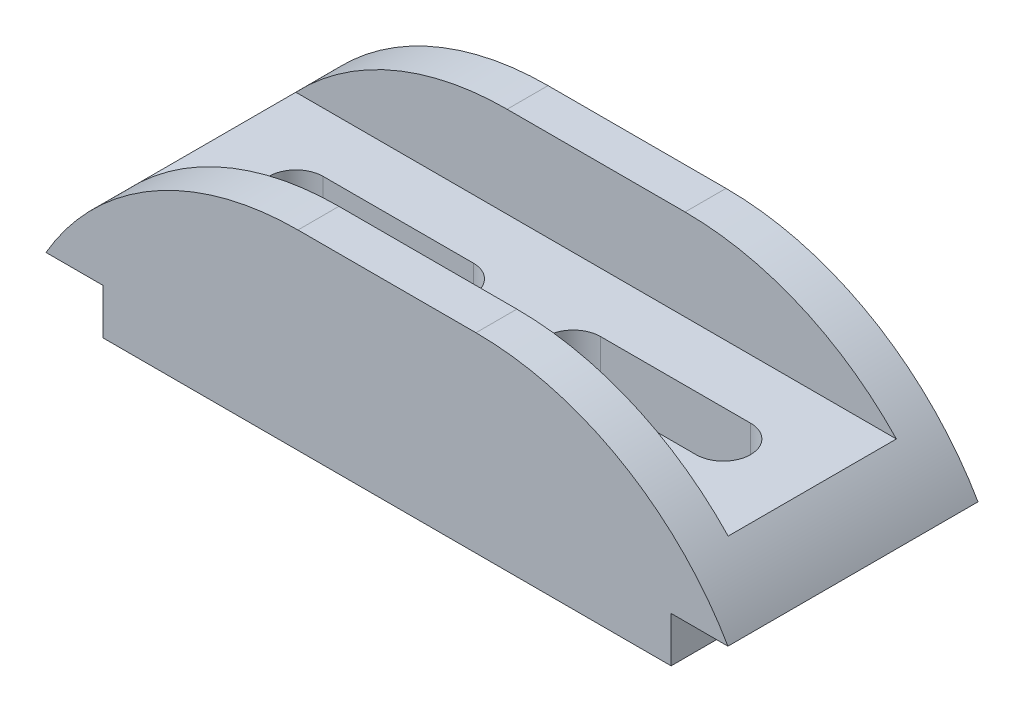
ISO-10303-21;
HEADER;
FILE_DESCRIPTION(('STEP AP214'),'2;1');
FILE_NAME('part.step','',(''),(''),'','','');
FILE_SCHEMA(('AUTOMOTIVE_DESIGN { 1 0 10303 214 1 1 1 1 }'));
ENDSEC;
DATA;
#1=APPLICATION_CONTEXT('core data for automotive mechanical design processes');
#2=APPLICATION_PROTOCOL_DEFINITION('international standard','automotive_design',2000,#1);
#3=PRODUCT_CONTEXT('',#1,'mechanical');
#4=PRODUCT('Part','Part','',(#3));
#5=PRODUCT_RELATED_PRODUCT_CATEGORY('part','',(#4));
#6=PRODUCT_DEFINITION_FORMATION('','',#4);
#7=PRODUCT_DEFINITION_CONTEXT('part definition',#1,'design');
#8=PRODUCT_DEFINITION('design','',#6,#7);
#9=PRODUCT_DEFINITION_SHAPE('','',#8);
#10=(LENGTH_UNIT() NAMED_UNIT(*) SI_UNIT(.MILLI.,.METRE.));
#11=(NAMED_UNIT(*) PLANE_ANGLE_UNIT() SI_UNIT($,.RADIAN.));
#12=(NAMED_UNIT(*) SI_UNIT($,.STERADIAN.) SOLID_ANGLE_UNIT());
#13=UNCERTAINTY_MEASURE_WITH_UNIT(LENGTH_MEASURE(1.E-05),#10,'distance_accuracy_value','');
#14=(GEOMETRIC_REPRESENTATION_CONTEXT(3) GLOBAL_UNCERTAINTY_ASSIGNED_CONTEXT((#13)) GLOBAL_UNIT_ASSIGNED_CONTEXT((#10,
#11,#12)) REPRESENTATION_CONTEXT('',''));
#15=CARTESIAN_POINT('',(0.,0.,0.));
#16=DIRECTION('',(0.,0.,1.));
#17=DIRECTION('',(1.,0.,0.));
#18=AXIS2_PLACEMENT_3D('',#15,#16,#17);
#19=CARTESIAN_POINT('',(-75.,21.,-55.));
#20=DIRECTION('',(0.,1.,0.));
#21=DIRECTION('',(0.,0.,1.));
#22=AXIS2_PLACEMENT_3D('',#19,#20,#21);
#23=PLANE('',#22);
#24=DIRECTION('',(0.,0.,-1.));
#25=VECTOR('',#24,1.);
#26=CARTESIAN_POINT('',(-19.5743741577959,21.,0.));
#27=LINE('',#26,#25);
#28=CARTESIAN_POINT('',(-19.5743741577959,21.,-55.));
#29=VERTEX_POINT('',#28);
#30=CARTESIAN_POINT('',(-19.5743741577959,21.,-46.));
#31=VERTEX_POINT('',#30);
#32=EDGE_CURVE('E299',#29,#31,#27,.F.);
#33=ORIENTED_EDGE('',*,*,#32,.T.);
#34=DIRECTION('',(1.,0.,0.));
#35=VECTOR('',#34,1.);
#36=CARTESIAN_POINT('',(-75.,21.,-46.));
#37=LINE('',#36,#35);
#38=CARTESIAN_POINT('',(19.5743741577959,21.,-46.));
#39=VERTEX_POINT('',#38);
#40=EDGE_CURVE('E208',#31,#39,#37,.T.);
#41=ORIENTED_EDGE('',*,*,#40,.T.);
#42=DIRECTION('',(0.,0.,1.));
#43=VECTOR('',#42,1.);
#44=CARTESIAN_POINT('',(19.5743741577959,21.,-55.));
#45=LINE('',#44,#43);
#46=CARTESIAN_POINT('',(19.5743741577959,21.,-55.));
#47=VERTEX_POINT('',#46);
#48=EDGE_CURVE('E284',#39,#47,#45,.F.);
#49=ORIENTED_EDGE('',*,*,#48,.T.);
#50=DIRECTION('',(-1.,0.,0.));
#51=VECTOR('',#50,1.);
#52=CARTESIAN_POINT('',(-75.,21.,-55.));
#53=LINE('',#52,#51);
#54=EDGE_CURVE('E265',#47,#29,#53,.T.);
#55=ORIENTED_EDGE('',*,*,#54,.T.);
#56=EDGE_LOOP('',(#33,#41,#49,#55));
#57=FACE_BOUND('',#56,.T.);
#58=ADVANCED_FACE('F39',(#57),#23,.T.);
#59=DIRECTION('',(1.,0.,0.));
#60=VECTOR('',#59,1.);
#61=CARTESIAN_POINT('',(-75.,21.,-9.));
#62=LINE('',#61,#60);
#63=CARTESIAN_POINT('',(-19.5743741577959,21.,-9.));
#64=VERTEX_POINT('',#63);
#65=CARTESIAN_POINT('',(19.5743741577959,21.,-8.99999999999999));
#66=VERTEX_POINT('',#65);
#67=EDGE_CURVE('E237',#64,#66,#62,.T.);
#68=ORIENTED_EDGE('',*,*,#67,.F.);
#69=CARTESIAN_POINT('',(-19.5743741577959,21.,0.));
#70=VERTEX_POINT('',#69);
#71=EDGE_CURVE('E297',#64,#70,#27,.F.);
#72=ORIENTED_EDGE('',*,*,#71,.T.);
#73=DIRECTION('',(-1.,0.,0.));
#74=VECTOR('',#73,1.);
#75=CARTESIAN_POINT('',(-75.,21.,0.));
#76=LINE('',#75,#74);
#77=CARTESIAN_POINT('',(19.5743741577959,21.,0.));
#78=VERTEX_POINT('',#77);
#79=EDGE_CURVE('E249',#78,#70,#76,.T.);
#80=ORIENTED_EDGE('',*,*,#79,.F.);
#81=EDGE_CURVE('E298',#78,#66,#45,.F.);
#82=ORIENTED_EDGE('',*,*,#81,.T.);
#83=EDGE_LOOP('',(#68,#72,#80,#82));
#84=FACE_BOUND('',#83,.T.);
#85=ADVANCED_FACE('F349',(#84),#23,.T.);
#86=CARTESIAN_POINT('',(62.5,-11.,-55.));
#87=DIRECTION('',(0.,-1.,0.));
#88=DIRECTION('',(0.,0.,-1.));
#89=AXIS2_PLACEMENT_3D('',#86,#87,#88);
#90=PLANE('',#89);
#91=DIRECTION('',(1.,0.,0.));
#92=VECTOR('',#91,1.);
#93=CARTESIAN_POINT('',(62.5,-11.,0.));
#94=LINE('',#93,#92);
#95=CARTESIAN_POINT('',(62.5,-11.,0.));
#96=VERTEX_POINT('',#95);
#97=CARTESIAN_POINT('',(75.,-11.,0.));
#98=VERTEX_POINT('',#97);
#99=EDGE_CURVE('E280',#96,#98,#94,.T.);
#100=ORIENTED_EDGE('',*,*,#99,.F.);
#101=DIRECTION('',(0.,0.,1.));
#102=VECTOR('',#101,1.);
#103=CARTESIAN_POINT('',(62.5,-11.,-55.));
#104=LINE('',#103,#102);
#105=CARTESIAN_POINT('',(62.5,-11.,-55.));
#106=VERTEX_POINT('',#105);
#107=EDGE_CURVE('E286',#106,#96,#104,.T.);
#108=ORIENTED_EDGE('',*,*,#107,.F.);
#109=DIRECTION('',(1.,0.,0.));
#110=VECTOR('',#109,1.);
#111=CARTESIAN_POINT('',(62.5,-11.,-55.));
#112=LINE('',#111,#110);
#113=CARTESIAN_POINT('',(75.,-11.,-55.));
#114=VERTEX_POINT('',#113);
#115=EDGE_CURVE('E259',#106,#114,#112,.T.);
#116=ORIENTED_EDGE('',*,*,#115,.T.);
#117=DIRECTION('',(0.,0.,1.));
#118=VECTOR('',#117,1.);
#119=CARTESIAN_POINT('',(75.,-11.,-55.));
#120=LINE('',#119,#118);
#121=EDGE_CURVE('E285',#114,#98,#120,.T.);
#122=ORIENTED_EDGE('',*,*,#121,.T.);
#123=EDGE_LOOP('',(#100,#108,#116,#122));
#124=FACE_BOUND('',#123,.T.);
#125=ADVANCED_FACE('F356',(#124),#90,.T.);
#126=CARTESIAN_POINT('',(62.5,-21.,-55.));
#127=DIRECTION('',(1.,0.,0.));
#128=DIRECTION('',(0.,0.,-1.));
#129=AXIS2_PLACEMENT_3D('',#126,#127,#128);
#130=PLANE('',#129);
#131=DIRECTION('',(0.,1.,0.));
#132=VECTOR('',#131,1.);
#133=CARTESIAN_POINT('',(62.5,-21.,0.));
#134=LINE('',#133,#132);
#135=CARTESIAN_POINT('',(62.5,-21.,0.));
#136=VERTEX_POINT('',#135);
#137=EDGE_CURVE('E273',#136,#96,#134,.T.);
#138=ORIENTED_EDGE('',*,*,#137,.F.);
#139=DIRECTION('',(0.,0.,1.));
#140=VECTOR('',#139,1.);
#141=CARTESIAN_POINT('',(62.5,-21.,-55.));
#142=LINE('',#141,#140);
#143=CARTESIAN_POINT('',(62.5,-21.,-55.));
#144=VERTEX_POINT('',#143);
#145=EDGE_CURVE('E288',#144,#136,#142,.T.);
#146=ORIENTED_EDGE('',*,*,#145,.F.);
#147=DIRECTION('',(0.,1.,0.));
#148=VECTOR('',#147,1.);
#149=CARTESIAN_POINT('',(62.5,-21.,-55.));
#150=LINE('',#149,#148);
#151=EDGE_CURVE('E258',#144,#106,#150,.T.);
#152=ORIENTED_EDGE('',*,*,#151,.T.);
#153=ORIENTED_EDGE('',*,*,#107,.T.);
#154=EDGE_LOOP('',(#138,#146,#152,#153));
#155=FACE_BOUND('',#154,.T.);
#156=ADVANCED_FACE('F365',(#155),#130,.T.);
#157=CARTESIAN_POINT('',(62.5,-21.,-55.));
#158=DIRECTION('',(0.,-1.,0.));
#159=DIRECTION('',(1.,0.,0.));
#160=AXIS2_PLACEMENT_3D('',#157,#158,#159);
#161=PLANE('',#160);
#162=CARTESIAN_POINT('',(-47.,-21.,-26.9775156815973));
#163=DIRECTION('',(0.,1.,0.));
#164=DIRECTION('',(0.,0.,1.));
#165=AXIS2_PLACEMENT_3D('',#162,#163,#164);
#166=CIRCLE('',#165,6.);
#167=CARTESIAN_POINT('',(-47.,-21.,-32.9775156815973));
#168=VERTEX_POINT('',#167);
#169=CARTESIAN_POINT('',(-47.,-21.,-20.9775156815973));
#170=VERTEX_POINT('',#169);
#171=EDGE_CURVE('E181',#168,#170,#166,.T.);
#172=ORIENTED_EDGE('',*,*,#171,.T.);
#173=DIRECTION('',(1.,0.,0.));
#174=VECTOR('',#173,1.);
#175=CARTESIAN_POINT('',(-47.,-21.,-20.9775156815973));
#176=LINE('',#175,#174);
#177=CARTESIAN_POINT('',(-14.,-21.,-20.9775156815973));
#178=VERTEX_POINT('',#177);
#179=EDGE_CURVE('E191',#170,#178,#176,.T.);
#180=ORIENTED_EDGE('',*,*,#179,.T.);
#181=CARTESIAN_POINT('',(-14.,-21.,-26.9775156815973));
#182=DIRECTION('',(0.,1.,0.));
#183=DIRECTION('',(0.,0.,1.));
#184=AXIS2_PLACEMENT_3D('',#181,#182,#183);
#185=CIRCLE('',#184,6.);
#186=CARTESIAN_POINT('',(-14.,-21.,-32.9775156815973));
#187=VERTEX_POINT('',#186);
#188=EDGE_CURVE('E53',#178,#187,#185,.T.);
#189=ORIENTED_EDGE('',*,*,#188,.T.);
#190=DIRECTION('',(-1.,0.,0.));
#191=VECTOR('',#190,1.);
#192=CARTESIAN_POINT('',(-47.,-21.,-32.9775156815973));
#193=LINE('',#192,#191);
#194=EDGE_CURVE('E186',#187,#168,#193,.T.);
#195=ORIENTED_EDGE('',*,*,#194,.T.);
#196=EDGE_LOOP('',(#172,#180,#189,#195));
#197=FACE_BOUND('',#196,.T.);
#198=CARTESIAN_POINT('',(14.,-21.,-26.9775156815973));
#199=DIRECTION('',(0.,1.,0.));
#200=DIRECTION('',(0.,0.,1.));
#201=AXIS2_PLACEMENT_3D('',#198,#199,#200);
#202=CIRCLE('',#201,6.);
#203=CARTESIAN_POINT('',(14.,-21.,-32.9775156815973));
#204=VERTEX_POINT('',#203);
#205=CARTESIAN_POINT('',(14.,-21.,-20.9775156815973));
#206=VERTEX_POINT('',#205);
#207=EDGE_CURVE('E196',#204,#206,#202,.T.);
#208=ORIENTED_EDGE('',*,*,#207,.T.);
#209=DIRECTION('',(1.,0.,0.));
#210=VECTOR('',#209,1.);
#211=CARTESIAN_POINT('',(14.,-21.,-20.9775156815973));
#212=LINE('',#211,#210);
#213=CARTESIAN_POINT('',(47.,-21.,-20.9775156815973));
#214=VERTEX_POINT('',#213);
#215=EDGE_CURVE('E203',#206,#214,#212,.T.);
#216=ORIENTED_EDGE('',*,*,#215,.T.);
#217=CARTESIAN_POINT('',(47.,-21.,-26.9775156815973));
#218=DIRECTION('',(0.,1.,0.));
#219=DIRECTION('',(0.,0.,1.));
#220=AXIS2_PLACEMENT_3D('',#217,#218,#219);
#221=CIRCLE('',#220,6.);
#222=CARTESIAN_POINT('',(47.,-21.,-32.9775156815973));
#223=VERTEX_POINT('',#222);
#224=EDGE_CURVE('E65',#214,#223,#221,.T.);
#225=ORIENTED_EDGE('',*,*,#224,.T.);
#226=DIRECTION('',(-1.,0.,0.));
#227=VECTOR('',#226,1.);
#228=CARTESIAN_POINT('',(14.,-21.,-32.9775156815973));
#229=LINE('',#228,#227);
#230=EDGE_CURVE('E214',#223,#204,#229,.T.);
#231=ORIENTED_EDGE('',*,*,#230,.T.);
#232=EDGE_LOOP('',(#208,#216,#225,#231));
#233=FACE_BOUND('',#232,.T.);
#234=DIRECTION('',(1.,0.,0.));
#235=VECTOR('',#234,1.);
#236=CARTESIAN_POINT('',(62.5,-21.,0.));
#237=LINE('',#236,#235);
#238=CARTESIAN_POINT('',(-62.5,-21.,0.));
#239=VERTEX_POINT('',#238);
#240=EDGE_CURVE('E271',#239,#136,#237,.T.);
#241=ORIENTED_EDGE('',*,*,#240,.F.);
#242=DIRECTION('',(0.,0.,1.));
#243=VECTOR('',#242,1.);
#244=CARTESIAN_POINT('',(-62.5,-21.,-55.));
#245=LINE('',#244,#243);
#246=CARTESIAN_POINT('',(-62.5,-21.,-55.));
#247=VERTEX_POINT('',#246);
#248=EDGE_CURVE('E289',#247,#239,#245,.T.);
#249=ORIENTED_EDGE('',*,*,#248,.F.);
#250=DIRECTION('',(1.,0.,0.));
#251=VECTOR('',#250,1.);
#252=CARTESIAN_POINT('',(62.5,-21.,-55.));
#253=LINE('',#252,#251);
#254=EDGE_CURVE('E251',#247,#144,#253,.T.);
#255=ORIENTED_EDGE('',*,*,#254,.T.);
#256=ORIENTED_EDGE('',*,*,#145,.T.);
#257=EDGE_LOOP('',(#241,#249,#255,#256));
#258=FACE_BOUND('',#257,.T.);
#259=ADVANCED_FACE('F194',(#197,#233,#258),#161,.T.);
#260=CARTESIAN_POINT('',(-62.5,-21.,-55.));
#261=DIRECTION('',(-1.,0.,0.));
#262=DIRECTION('',(0.,0.,1.));
#263=AXIS2_PLACEMENT_3D('',#260,#261,#262);
#264=PLANE('',#263);
#265=DIRECTION('',(0.,-1.,0.));
#266=VECTOR('',#265,1.);
#267=CARTESIAN_POINT('',(-62.5,-21.,0.));
#268=LINE('',#267,#266);
#269=CARTESIAN_POINT('',(-62.5,-11.,0.));
#270=VERTEX_POINT('',#269);
#271=EDGE_CURVE('E268',#270,#239,#268,.T.);
#272=ORIENTED_EDGE('',*,*,#271,.F.);
#273=DIRECTION('',(0.,0.,1.));
#274=VECTOR('',#273,1.);
#275=CARTESIAN_POINT('',(-62.5,-11.,-55.));
#276=LINE('',#275,#274);
#277=CARTESIAN_POINT('',(-62.5,-11.,-55.));
#278=VERTEX_POINT('',#277);
#279=EDGE_CURVE('E295',#278,#270,#276,.T.);
#280=ORIENTED_EDGE('',*,*,#279,.F.);
#281=DIRECTION('',(0.,-1.,0.));
#282=VECTOR('',#281,1.);
#283=CARTESIAN_POINT('',(-62.5,-21.,-55.));
#284=LINE('',#283,#282);
#285=EDGE_CURVE('E247',#278,#247,#284,.T.);
#286=ORIENTED_EDGE('',*,*,#285,.T.);
#287=ORIENTED_EDGE('',*,*,#248,.T.);
#288=EDGE_LOOP('',(#272,#280,#286,#287));
#289=FACE_BOUND('',#288,.T.);
#290=ADVANCED_FACE('F371',(#289),#264,.T.);
#291=CARTESIAN_POINT('',(-62.5,-11.,-55.));
#292=DIRECTION('',(0.,-1.,0.));
#293=DIRECTION('',(0.,0.,-1.));
#294=AXIS2_PLACEMENT_3D('',#291,#292,#293);
#295=PLANE('',#294);
#296=DIRECTION('',(1.,0.,0.));
#297=VECTOR('',#296,1.);
#298=CARTESIAN_POINT('',(-62.5,-11.,0.));
#299=LINE('',#298,#297);
#300=CARTESIAN_POINT('',(-75.,-11.,0.));
#301=VERTEX_POINT('',#300);
#302=EDGE_CURVE('E244',#301,#270,#299,.T.);
#303=ORIENTED_EDGE('',*,*,#302,.F.);
#304=DIRECTION('',(0.,0.,1.));
#305=VECTOR('',#304,1.);
#306=CARTESIAN_POINT('',(-75.,-11.,-55.));
#307=LINE('',#306,#305);
#308=CARTESIAN_POINT('',(-75.,-11.,-55.));
#309=VERTEX_POINT('',#308);
#310=EDGE_CURVE('E264',#309,#301,#307,.T.);
#311=ORIENTED_EDGE('',*,*,#310,.F.);
#312=DIRECTION('',(1.,0.,0.));
#313=VECTOR('',#312,1.);
#314=CARTESIAN_POINT('',(-62.5,-11.,-55.));
#315=LINE('',#314,#313);
#316=EDGE_CURVE('E246',#309,#278,#315,.T.);
#317=ORIENTED_EDGE('',*,*,#316,.T.);
#318=ORIENTED_EDGE('',*,*,#279,.T.);
#319=EDGE_LOOP('',(#303,#311,#317,#318));
#320=FACE_BOUND('',#319,.T.);
#321=ADVANCED_FACE('F372',(#320),#295,.T.);
#322=CARTESIAN_POINT('',(0.,0.,-55.));
#323=DIRECTION('',(0.,0.,-1.));
#324=DIRECTION('',(-1.,0.,0.));
#325=AXIS2_PLACEMENT_3D('',#322,#323,#324);
#326=PLANE('',#325);
#327=ORIENTED_EDGE('',*,*,#316,.F.);
#328=CARTESIAN_POINT('',(-19.5743741577959,-43.,-55.));
#329=DIRECTION('',(0.,0.,-1.));
#330=DIRECTION('',(-1.,0.,0.));
#331=AXIS2_PLACEMENT_3D('',#328,#329,#330);
#332=CIRCLE('',#331,64.);
#333=EDGE_CURVE('E310',#309,#29,#332,.T.);
#334=ORIENTED_EDGE('',*,*,#333,.T.);
#335=ORIENTED_EDGE('',*,*,#54,.F.);
#336=CARTESIAN_POINT('',(19.5743741577959,-43.,-55.));
#337=DIRECTION('',(0.,0.,-1.));
#338=DIRECTION('',(-1.,0.,0.));
#339=AXIS2_PLACEMENT_3D('',#336,#337,#338);
#340=CIRCLE('',#339,64.);
#341=EDGE_CURVE('E307',#47,#114,#340,.T.);
#342=ORIENTED_EDGE('',*,*,#341,.T.);
#343=ORIENTED_EDGE('',*,*,#115,.F.);
#344=ORIENTED_EDGE('',*,*,#151,.F.);
#345=ORIENTED_EDGE('',*,*,#254,.F.);
#346=ORIENTED_EDGE('',*,*,#285,.F.);
#347=EDGE_LOOP('',(#327,#334,#335,#342,#343,#344,#345,#346));
#348=FACE_BOUND('',#347,.T.);
#349=ADVANCED_FACE('F380',(#348),#326,.T.);
#350=CARTESIAN_POINT('',(0.,0.,0.));
#351=DIRECTION('',(0.,0.,-1.));
#352=DIRECTION('',(-1.,0.,0.));
#353=AXIS2_PLACEMENT_3D('',#350,#351,#352);
#354=PLANE('',#353);
#355=ORIENTED_EDGE('',*,*,#79,.T.);
#356=CARTESIAN_POINT('',(-19.5743741577959,-43.,0.));
#357=DIRECTION('',(0.,0.,-1.));
#358=DIRECTION('',(-1.,0.,0.));
#359=AXIS2_PLACEMENT_3D('',#356,#357,#358);
#360=CIRCLE('',#359,64.);
#361=EDGE_CURVE('E304',#70,#301,#360,.F.);
#362=ORIENTED_EDGE('',*,*,#361,.T.);
#363=ORIENTED_EDGE('',*,*,#302,.T.);
#364=ORIENTED_EDGE('',*,*,#271,.T.);
#365=ORIENTED_EDGE('',*,*,#240,.T.);
#366=ORIENTED_EDGE('',*,*,#137,.T.);
#367=ORIENTED_EDGE('',*,*,#99,.T.);
#368=CARTESIAN_POINT('',(19.5743741577959,-43.,0.));
#369=DIRECTION('',(0.,0.,-1.));
#370=DIRECTION('',(-1.,0.,0.));
#371=AXIS2_PLACEMENT_3D('',#368,#369,#370);
#372=CIRCLE('',#371,64.);
#373=EDGE_CURVE('E303',#98,#78,#372,.F.);
#374=ORIENTED_EDGE('',*,*,#373,.T.);
#375=EDGE_LOOP('',(#355,#362,#363,#364,#365,#366,#367,#374));
#376=FACE_BOUND('',#375,.T.);
#377=ADVANCED_FACE('F359',(#376),#354,.F.);
#378=CARTESIAN_POINT('',(-19.5743741577959,-43.,-55.));
#379=DIRECTION('',(0.,0.,1.));
#380=DIRECTION('',(1.,0.,0.));
#381=AXIS2_PLACEMENT_3D('',#378,#379,#380);
#382=CYLINDRICAL_SURFACE('',#381,64.);
#383=CARTESIAN_POINT('',(-19.5743741577959,-43.,-46.));
#384=DIRECTION('',(0.,0.,-1.));
#385=DIRECTION('',(-1.,0.,0.));
#386=AXIS2_PLACEMENT_3D('',#383,#384,#385);
#387=CIRCLE('',#386,64.);
#388=CARTESIAN_POINT('',(-66.050174312285,0.999999999999997,-46.));
#389=VERTEX_POINT('',#388);
#390=EDGE_CURVE('E241',#31,#389,#387,.F.);
#391=ORIENTED_EDGE('',*,*,#390,.F.);
#392=ORIENTED_EDGE('',*,*,#32,.F.);
#393=ORIENTED_EDGE('',*,*,#333,.F.);
#394=ORIENTED_EDGE('',*,*,#310,.T.);
#395=ORIENTED_EDGE('',*,*,#361,.F.);
#396=ORIENTED_EDGE('',*,*,#71,.F.);
#397=CARTESIAN_POINT('',(-19.5743741577959,-43.,-9.00000000000001));
#398=DIRECTION('',(0.,0.,1.));
#399=DIRECTION('',(0.,-1.,0.));
#400=AXIS2_PLACEMENT_3D('',#397,#398,#399);
#401=CIRCLE('',#400,64.);
#402=CARTESIAN_POINT('',(-66.050174312285,0.999999999999994,-9.));
#403=VERTEX_POINT('',#402);
#404=EDGE_CURVE('E235',#403,#64,#401,.F.);
#405=ORIENTED_EDGE('',*,*,#404,.F.);
#406=DIRECTION('',(0.,0.,1.));
#407=VECTOR('',#406,1.);
#408=CARTESIAN_POINT('',(-66.050174312285,0.999999999999994,-55.));
#409=LINE('',#408,#407);
#410=EDGE_CURVE('E243',#389,#403,#409,.T.);
#411=ORIENTED_EDGE('',*,*,#410,.F.);
#412=EDGE_LOOP('',(#391,#392,#393,#394,#395,#396,#405,#411));
#413=FACE_BOUND('',#412,.T.);
#414=ADVANCED_FACE('F377',(#413),#382,.T.);
#415=CARTESIAN_POINT('',(19.5743741577959,-43.,-55.));
#416=DIRECTION('',(0.,0.,-1.));
#417=DIRECTION('',(-1.,0.,0.));
#418=AXIS2_PLACEMENT_3D('',#415,#416,#417);
#419=CYLINDRICAL_SURFACE('',#418,64.);
#420=CARTESIAN_POINT('',(19.5743741577959,-43.,-46.));
#421=DIRECTION('',(0.,0.,-1.));
#422=DIRECTION('',(-1.,0.,0.));
#423=AXIS2_PLACEMENT_3D('',#420,#421,#422);
#424=CIRCLE('',#423,64.);
#425=CARTESIAN_POINT('',(66.0501743122849,0.999999999999997,-46.));
#426=VERTEX_POINT('',#425);
#427=EDGE_CURVE('E312',#426,#39,#424,.F.);
#428=ORIENTED_EDGE('',*,*,#427,.F.);
#429=DIRECTION('',(0.,0.,-1.));
#430=VECTOR('',#429,1.);
#431=CARTESIAN_POINT('',(66.0501743122849,0.999999999999994,-55.));
#432=LINE('',#431,#430);
#433=CARTESIAN_POINT('',(66.0501743122849,0.999999999999994,-9.));
#434=VERTEX_POINT('',#433);
#435=EDGE_CURVE('E311',#434,#426,#432,.T.);
#436=ORIENTED_EDGE('',*,*,#435,.F.);
#437=CARTESIAN_POINT('',(19.5743741577959,-43.,-9.00000000000001));
#438=DIRECTION('',(0.,0.,1.));
#439=DIRECTION('',(0.,-1.,0.));
#440=AXIS2_PLACEMENT_3D('',#437,#438,#439);
#441=CIRCLE('',#440,64.);
#442=EDGE_CURVE('E313',#66,#434,#441,.F.);
#443=ORIENTED_EDGE('',*,*,#442,.F.);
#444=ORIENTED_EDGE('',*,*,#81,.F.);
#445=ORIENTED_EDGE('',*,*,#373,.F.);
#446=ORIENTED_EDGE('',*,*,#121,.F.);
#447=ORIENTED_EDGE('',*,*,#341,.F.);
#448=ORIENTED_EDGE('',*,*,#48,.F.);
#449=EDGE_LOOP('',(#428,#436,#443,#444,#445,#446,#447,#448));
#450=FACE_BOUND('',#449,.T.);
#451=ADVANCED_FACE('F41',(#450),#419,.T.);
#452=CARTESIAN_POINT('',(-75.,21.,-46.));
#453=DIRECTION('',(0.,0.,-1.));
#454=DIRECTION('',(-1.,0.,0.));
#455=AXIS2_PLACEMENT_3D('',#452,#453,#454);
#456=PLANE('',#455);
#457=ORIENTED_EDGE('',*,*,#390,.T.);
#458=DIRECTION('',(1.,0.,0.));
#459=VECTOR('',#458,1.);
#460=CARTESIAN_POINT('',(-75.,0.999999999999997,-46.));
#461=LINE('',#460,#459);
#462=EDGE_CURVE('E227',#389,#426,#461,.T.);
#463=ORIENTED_EDGE('',*,*,#462,.T.);
#464=ORIENTED_EDGE('',*,*,#427,.T.);
#465=ORIENTED_EDGE('',*,*,#40,.F.);
#466=EDGE_LOOP('',(#457,#463,#464,#465));
#467=FACE_BOUND('',#466,.T.);
#468=ADVANCED_FACE('F384',(#467),#456,.F.);
#469=CARTESIAN_POINT('',(-75.,0.999999999999997,-9.));
#470=DIRECTION('',(0.,-1.,0.));
#471=DIRECTION('',(0.,0.,-1.));
#472=AXIS2_PLACEMENT_3D('',#469,#470,#471);
#473=PLANE('',#472);
#474=DIRECTION('',(-1.,0.,0.));
#475=VECTOR('',#474,1.);
#476=CARTESIAN_POINT('',(-75.,0.999999999999997,-20.9775156815973));
#477=LINE('',#476,#475);
#478=CARTESIAN_POINT('',(-14.,0.999999999999997,-20.9775156815973));
#479=VERTEX_POINT('',#478);
#480=CARTESIAN_POINT('',(-47.,0.999999999999997,-20.9775156815973));
#481=VERTEX_POINT('',#480);
#482=EDGE_CURVE('E328',#479,#481,#477,.T.);
#483=ORIENTED_EDGE('',*,*,#482,.T.);
#484=CARTESIAN_POINT('',(-47.,0.999999999999997,-26.9775156815973));
#485=DIRECTION('',(0.,-1.,0.));
#486=DIRECTION('',(0.,0.,-1.));
#487=AXIS2_PLACEMENT_3D('',#484,#485,#486);
#488=CIRCLE('',#487,6.);
#489=CARTESIAN_POINT('',(-47.,0.999999999999997,-32.9775156815973));
#490=VERTEX_POINT('',#489);
#491=EDGE_CURVE('E11',#481,#490,#488,.T.);
#492=ORIENTED_EDGE('',*,*,#491,.T.);
#493=DIRECTION('',(1.,0.,0.));
#494=VECTOR('',#493,1.);
#495=CARTESIAN_POINT('',(-75.,0.999999999999997,-32.9775156815973));
#496=LINE('',#495,#494);
#497=CARTESIAN_POINT('',(-14.,0.999999999999997,-32.9775156815973));
#498=VERTEX_POINT('',#497);
#499=EDGE_CURVE('E50',#490,#498,#496,.T.);
#500=ORIENTED_EDGE('',*,*,#499,.T.);
#501=CARTESIAN_POINT('',(-14.,0.999999999999997,-26.9775156815973));
#502=DIRECTION('',(0.,-1.,0.));
#503=DIRECTION('',(0.,0.,-1.));
#504=AXIS2_PLACEMENT_3D('',#501,#502,#503);
#505=CIRCLE('',#504,6.);
#506=EDGE_CURVE('E332',#498,#479,#505,.T.);
#507=ORIENTED_EDGE('',*,*,#506,.T.);
#508=EDGE_LOOP('',(#483,#492,#500,#507));
#509=FACE_BOUND('',#508,.T.);
#510=DIRECTION('',(-1.,0.,0.));
#511=VECTOR('',#510,1.);
#512=CARTESIAN_POINT('',(-75.,0.999999999999997,-20.9775156815973));
#513=LINE('',#512,#511);
#514=CARTESIAN_POINT('',(47.,0.999999999999997,-20.9775156815973));
#515=VERTEX_POINT('',#514);
#516=CARTESIAN_POINT('',(14.,0.999999999999997,-20.9775156815973));
#517=VERTEX_POINT('',#516);
#518=EDGE_CURVE('E320',#515,#517,#513,.T.);
#519=ORIENTED_EDGE('',*,*,#518,.T.);
#520=CARTESIAN_POINT('',(14.,0.999999999999997,-26.9775156815973));
#521=DIRECTION('',(0.,-1.,0.));
#522=DIRECTION('',(0.,0.,-1.));
#523=AXIS2_PLACEMENT_3D('',#520,#521,#522);
#524=CIRCLE('',#523,6.);
#525=CARTESIAN_POINT('',(14.,0.999999999999997,-32.9775156815973));
#526=VERTEX_POINT('',#525);
#527=EDGE_CURVE('E326',#517,#526,#524,.T.);
#528=ORIENTED_EDGE('',*,*,#527,.T.);
#529=DIRECTION('',(1.,0.,0.));
#530=VECTOR('',#529,1.);
#531=CARTESIAN_POINT('',(-75.,0.999999999999997,-32.9775156815973));
#532=LINE('',#531,#530);
#533=CARTESIAN_POINT('',(47.,0.999999999999997,-32.9775156815973));
#534=VERTEX_POINT('',#533);
#535=EDGE_CURVE('E323',#526,#534,#532,.T.);
#536=ORIENTED_EDGE('',*,*,#535,.T.);
#537=CARTESIAN_POINT('',(47.,0.999999999999997,-26.9775156815973));
#538=DIRECTION('',(0.,-1.,0.));
#539=DIRECTION('',(0.,0.,-1.));
#540=AXIS2_PLACEMENT_3D('',#537,#538,#539);
#541=CIRCLE('',#540,6.);
#542=EDGE_CURVE('E319',#534,#515,#541,.T.);
#543=ORIENTED_EDGE('',*,*,#542,.T.);
#544=EDGE_LOOP('',(#519,#528,#536,#543));
#545=FACE_BOUND('',#544,.T.);
#546=ORIENTED_EDGE('',*,*,#410,.T.);
#547=DIRECTION('',(1.,0.,0.));
#548=VECTOR('',#547,1.);
#549=CARTESIAN_POINT('',(-75.,0.999999999999997,-9.));
#550=LINE('',#549,#548);
#551=EDGE_CURVE('E233',#403,#434,#550,.T.);
#552=ORIENTED_EDGE('',*,*,#551,.T.);
#553=ORIENTED_EDGE('',*,*,#435,.T.);
#554=ORIENTED_EDGE('',*,*,#462,.F.);
#555=EDGE_LOOP('',(#546,#552,#553,#554));
#556=FACE_BOUND('',#555,.T.);
#557=ADVANCED_FACE('F333',(#509,#545,#556),#473,.F.);
#558=CARTESIAN_POINT('',(-75.,21.,-9.));
#559=DIRECTION('',(0.,0.,1.));
#560=DIRECTION('',(0.,-1.,0.));
#561=AXIS2_PLACEMENT_3D('',#558,#559,#560);
#562=PLANE('',#561);
#563=ORIENTED_EDGE('',*,*,#404,.T.);
#564=ORIENTED_EDGE('',*,*,#67,.T.);
#565=ORIENTED_EDGE('',*,*,#442,.T.);
#566=ORIENTED_EDGE('',*,*,#551,.F.);
#567=EDGE_LOOP('',(#563,#564,#565,#566));
#568=FACE_BOUND('',#567,.T.);
#569=ADVANCED_FACE('F423',(#568),#562,.F.);
#570=CARTESIAN_POINT('',(14.,-21.,-26.9775156815973));
#571=DIRECTION('',(0.,1.,0.));
#572=DIRECTION('',(0.,0.,1.));
#573=AXIS2_PLACEMENT_3D('',#570,#571,#572);
#574=CYLINDRICAL_SURFACE('',#573,6.);
#575=DIRECTION('',(0.,1.,0.));
#576=VECTOR('',#575,1.);
#577=CARTESIAN_POINT('',(14.,-21.,-20.9775156815973));
#578=LINE('',#577,#576);
#579=EDGE_CURVE('E213',#206,#517,#578,.T.);
#580=ORIENTED_EDGE('',*,*,#579,.F.);
#581=ORIENTED_EDGE('',*,*,#207,.F.);
#582=DIRECTION('',(0.,1.,0.));
#583=VECTOR('',#582,1.);
#584=CARTESIAN_POINT('',(14.,-21.,-32.9775156815973));
#585=LINE('',#584,#583);
#586=EDGE_CURVE('E222',#204,#526,#585,.T.);
#587=ORIENTED_EDGE('',*,*,#586,.T.);
#588=ORIENTED_EDGE('',*,*,#527,.F.);
#589=EDGE_LOOP('',(#580,#581,#587,#588));
#590=FACE_BOUND('',#589,.T.);
#591=ADVANCED_FACE('F474',(#590),#574,.F.);
#592=CARTESIAN_POINT('',(14.,-21.,-32.9775156815973));
#593=DIRECTION('',(0.,0.,-1.));
#594=DIRECTION('',(-1.,0.,0.));
#595=AXIS2_PLACEMENT_3D('',#592,#593,#594);
#596=PLANE('',#595);
#597=ORIENTED_EDGE('',*,*,#586,.F.);
#598=ORIENTED_EDGE('',*,*,#230,.F.);
#599=DIRECTION('',(0.,1.,0.));
#600=VECTOR('',#599,1.);
#601=CARTESIAN_POINT('',(47.,-21.,-32.9775156815973));
#602=LINE('',#601,#600);
#603=EDGE_CURVE('E217',#223,#534,#602,.T.);
#604=ORIENTED_EDGE('',*,*,#603,.T.);
#605=ORIENTED_EDGE('',*,*,#535,.F.);
#606=EDGE_LOOP('',(#597,#598,#604,#605));
#607=FACE_BOUND('',#606,.T.);
#608=ADVANCED_FACE('F485',(#607),#596,.F.);
#609=CARTESIAN_POINT('',(47.,-21.,-26.9775156815973));
#610=DIRECTION('',(0.,1.,0.));
#611=DIRECTION('',(0.,0.,1.));
#612=AXIS2_PLACEMENT_3D('',#609,#610,#611);
#613=CYLINDRICAL_SURFACE('',#612,6.);
#614=ORIENTED_EDGE('',*,*,#603,.F.);
#615=ORIENTED_EDGE('',*,*,#224,.F.);
#616=DIRECTION('',(0.,1.,0.));
#617=VECTOR('',#616,1.);
#618=CARTESIAN_POINT('',(47.,-21.,-20.9775156815973));
#619=LINE('',#618,#617);
#620=EDGE_CURVE('E216',#214,#515,#619,.T.);
#621=ORIENTED_EDGE('',*,*,#620,.T.);
#622=ORIENTED_EDGE('',*,*,#542,.F.);
#623=EDGE_LOOP('',(#614,#615,#621,#622));
#624=FACE_BOUND('',#623,.T.);
#625=ADVANCED_FACE('F495',(#624),#613,.F.);
#626=CARTESIAN_POINT('',(14.,-21.,-20.9775156815973));
#627=DIRECTION('',(0.,0.,1.));
#628=DIRECTION('',(1.,0.,0.));
#629=AXIS2_PLACEMENT_3D('',#626,#627,#628);
#630=PLANE('',#629);
#631=ORIENTED_EDGE('',*,*,#620,.F.);
#632=ORIENTED_EDGE('',*,*,#215,.F.);
#633=ORIENTED_EDGE('',*,*,#579,.T.);
#634=ORIENTED_EDGE('',*,*,#518,.F.);
#635=EDGE_LOOP('',(#631,#632,#633,#634));
#636=FACE_BOUND('',#635,.T.);
#637=ADVANCED_FACE('F505',(#636),#630,.F.);
#638=CARTESIAN_POINT('',(-47.,-21.,-26.9775156815973));
#639=DIRECTION('',(0.,1.,0.));
#640=DIRECTION('',(0.,0.,1.));
#641=AXIS2_PLACEMENT_3D('',#638,#639,#640);
#642=CYLINDRICAL_SURFACE('',#641,6.);
#643=DIRECTION('',(0.,1.,0.));
#644=VECTOR('',#643,1.);
#645=CARTESIAN_POINT('',(-47.,-21.,-20.9775156815973));
#646=LINE('',#645,#644);
#647=EDGE_CURVE('E178',#170,#481,#646,.T.);
#648=ORIENTED_EDGE('',*,*,#647,.F.);
#649=ORIENTED_EDGE('',*,*,#171,.F.);
#650=DIRECTION('',(0.,1.,0.));
#651=VECTOR('',#650,1.);
#652=CARTESIAN_POINT('',(-47.,-21.,-32.9775156815973));
#653=LINE('',#652,#651);
#654=EDGE_CURVE('E206',#168,#490,#653,.T.);
#655=ORIENTED_EDGE('',*,*,#654,.T.);
#656=ORIENTED_EDGE('',*,*,#491,.F.);
#657=EDGE_LOOP('',(#648,#649,#655,#656));
#658=FACE_BOUND('',#657,.T.);
#659=ADVANCED_FACE('F179',(#658),#642,.F.);
#660=CARTESIAN_POINT('',(-47.,-21.,-32.9775156815973));
#661=DIRECTION('',(0.,0.,-1.));
#662=DIRECTION('',(-1.,0.,0.));
#663=AXIS2_PLACEMENT_3D('',#660,#661,#662);
#664=PLANE('',#663);
#665=ORIENTED_EDGE('',*,*,#654,.F.);
#666=ORIENTED_EDGE('',*,*,#194,.F.);
#667=DIRECTION('',(0.,1.,0.));
#668=VECTOR('',#667,1.);
#669=CARTESIAN_POINT('',(-14.,-21.,-32.9775156815973));
#670=LINE('',#669,#668);
#671=EDGE_CURVE('E207',#187,#498,#670,.T.);
#672=ORIENTED_EDGE('',*,*,#671,.T.);
#673=ORIENTED_EDGE('',*,*,#499,.F.);
#674=EDGE_LOOP('',(#665,#666,#672,#673));
#675=FACE_BOUND('',#674,.T.);
#676=ADVANCED_FACE('F336',(#675),#664,.F.);
#677=CARTESIAN_POINT('',(-14.,-21.,-26.9775156815973));
#678=DIRECTION('',(0.,1.,0.));
#679=DIRECTION('',(0.,0.,1.));
#680=AXIS2_PLACEMENT_3D('',#677,#678,#679);
#681=CYLINDRICAL_SURFACE('',#680,6.);
#682=ORIENTED_EDGE('',*,*,#671,.F.);
#683=ORIENTED_EDGE('',*,*,#188,.F.);
#684=DIRECTION('',(0.,1.,0.));
#685=VECTOR('',#684,1.);
#686=CARTESIAN_POINT('',(-14.,-21.,-20.9775156815973));
#687=LINE('',#686,#685);
#688=EDGE_CURVE('E190',#178,#479,#687,.T.);
#689=ORIENTED_EDGE('',*,*,#688,.T.);
#690=ORIENTED_EDGE('',*,*,#506,.F.);
#691=EDGE_LOOP('',(#682,#683,#689,#690));
#692=FACE_BOUND('',#691,.T.);
#693=ADVANCED_FACE('F337',(#692),#681,.F.);
#694=CARTESIAN_POINT('',(-47.,-21.,-20.9775156815973));
#695=DIRECTION('',(0.,0.,1.));
#696=DIRECTION('',(1.,0.,0.));
#697=AXIS2_PLACEMENT_3D('',#694,#695,#696);
#698=PLANE('',#697);
#699=ORIENTED_EDGE('',*,*,#688,.F.);
#700=ORIENTED_EDGE('',*,*,#179,.F.);
#701=ORIENTED_EDGE('',*,*,#647,.T.);
#702=ORIENTED_EDGE('',*,*,#482,.F.);
#703=EDGE_LOOP('',(#699,#700,#701,#702));
#704=FACE_BOUND('',#703,.T.);
#705=ADVANCED_FACE('F195',(#704),#698,.F.);
#706=CLOSED_SHELL('',(#58,#85,#125,#156,#259,#290,#321,#349,#377,#414,#451,#468,#557,#569,#591,
#608,#625,#637,#659,#676,#693,#705));
#707=MANIFOLD_SOLID_BREP('B2',#706);
#708=ADVANCED_BREP_SHAPE_REPRESENTATION('',(#18,#707),#14);
#709=SHAPE_DEFINITION_REPRESENTATION(#9,#708);
ENDSEC;
END-ISO-10303-21;
